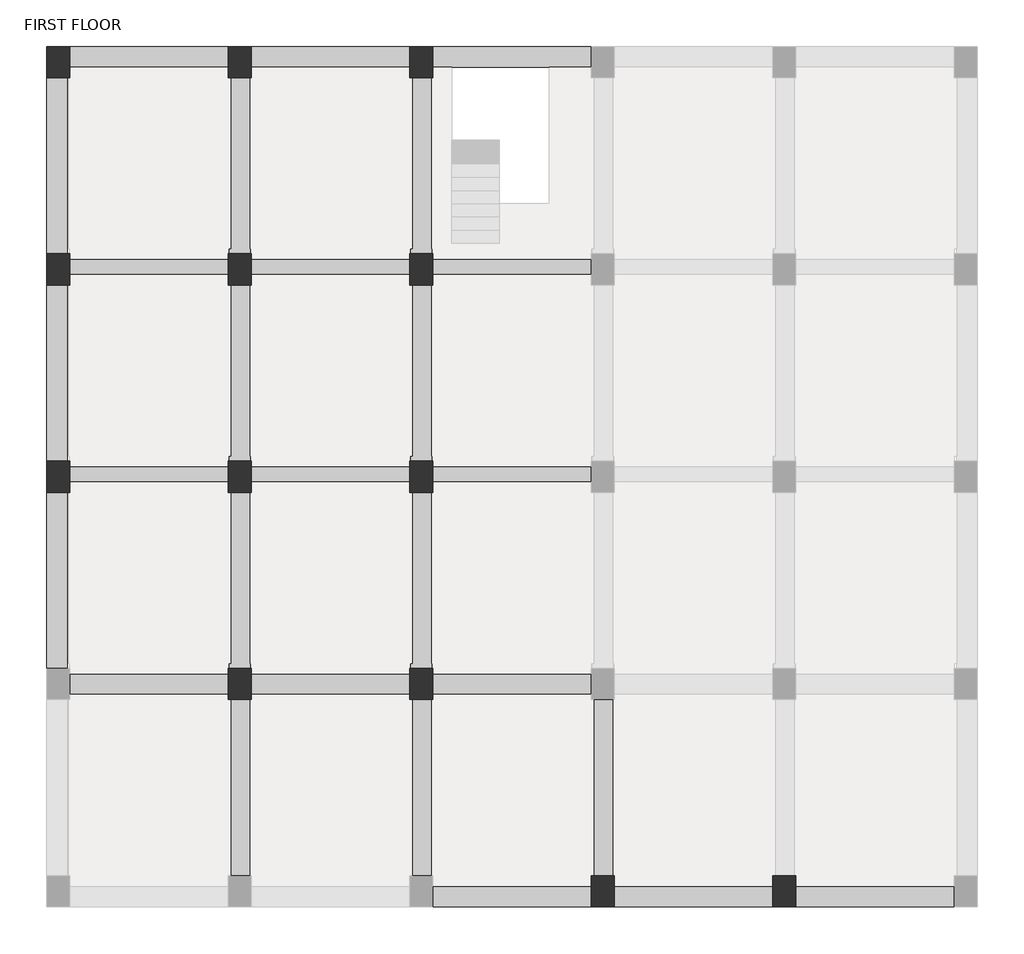
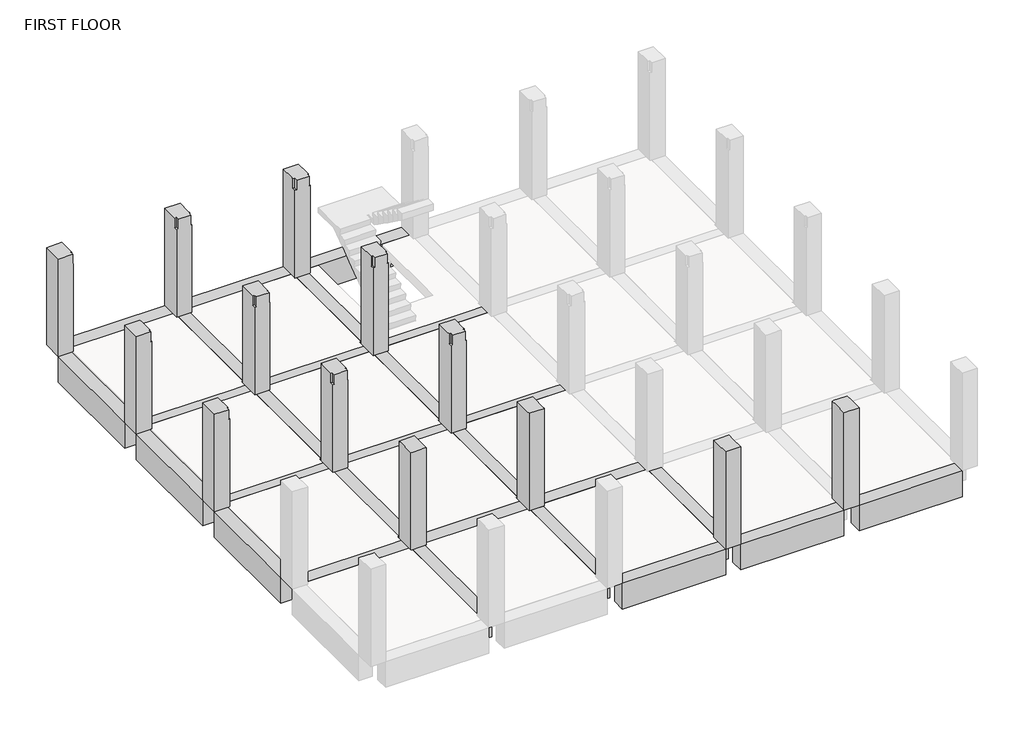
# One storey, part 3 of 4: 27 beams, 13 columns.
"""IFC4 building model written with IfcOpenShell, lengths in millimetres."""

from ifc_helpers import new_model, si_unit, frame, origin, place, context, project, spatial, polyline, outline, extrude, faceted_brep, element, save

model = new_model("IFC4")

# Units and contexts
model_context = context("Model", 3, world=origin())
ifc_project = project(units=[si_unit("LENGTHUNIT", "METRE", prefix="MILLI")], contexts=[model_context])

# Site, building, storey
site = spatial("IfcSite", under=ifc_project)
building = spatial("IfcBuilding", under=site)
storey = spatial("IfcBuildingStorey", under=building, Name="FIRST FLOOR", Elevation=3048.0)

# Beams
placement = place(None, origin())
element("IfcBeam", 1, ObjectType="M_Concrete-Rectangular Beam : 400 x 800mm", at=placement, inside=storey, context=model_context, shape_type="Brep", body=[
    faceted_brep([(4855.1115906, 3503.1212443, 3048.0), (4855.1115906, 3103.1212443, 3048.0), (7905.1115906, 3103.1212443, 3048.0), (7905.1115906, 3503.1212443, 3048.0), (4855.1115906, 3503.1212443, 2248.0), (4855.1115906, 3503.1212443, 2748.0), (7905.1115906, 3503.1212443, 2748.0), (7905.1115906, 3503.1212443, 2248.0), (4855.1115906, 3103.1212443, 2248.0), (7905.1115906, 3103.1212443, 2248.0)], [[[0, 1, 2, 3]], [[4, 5, 0, 3, 6, 7]], [[8, 4, 7, 9]], [[1, 8, 9, 2]], [[1, 0, 5, 4, 8]], [[3, 2, 9, 7, 6]]]),
])
element("IfcBeam", 2, ObjectType="M_Concrete-Rectangular Beam : 400 x 800mm", at=placement, inside=storey, context=model_context, shape_type="Brep", body=[
    faceted_brep([(1355.1115906, 3503.1212443, 3048.0), (1355.1115906, 3103.1212443, 3048.0), (4405.1115906, 3103.1212443, 3048.0), (4405.1115906, 3503.1212443, 3048.0), (1355.1115906, 3503.1212443, 2248.0), (1355.1115906, 3503.1212443, 2748.0), (4405.1115906, 3503.1212443, 2748.0), (4405.1115906, 3503.1212443, 2248.0), (1355.1115906, 3103.1212443, 2248.0), (4405.1115906, 3103.1212443, 2248.0)], [[[0, 1, 2, 3]], [[4, 5, 0, 3, 6, 7]], [[8, 4, 7, 9]], [[1, 8, 9, 2]], [[1, 0, 5, 4, 8]], [[3, 2, 9, 7, 6]]]),
])
element("IfcBeam", 3, ObjectType="M_Concrete-Rectangular Beam : 400 x 800mm", at=placement, inside=storey, context=model_context, shape_type="Brep", body=[
    faceted_brep([(-2144.8884094, 3503.1212443, 3048.0), (-2144.8884094, 3103.1212443, 3048.0), (905.1115906, 3103.1212443, 3048.0), (905.1115906, 3503.1212443, 3048.0), (-2144.8884094, 3503.1212443, 2248.0), (-2144.8884094, 3503.1212443, 2748.0), (905.1115906, 3503.1212443, 2748.0), (905.1115906, 3503.1212443, 2248.0), (-2144.8884094, 3103.1212443, 2248.0), (905.1115906, 3103.1212443, 2248.0)], [[[0, 1, 2, 3]], [[4, 5, 0, 3, 6, 7]], [[8, 4, 7, 9]], [[1, 8, 9, 2]], [[1, 0, 5, 4, 8]], [[3, 2, 9, 7, 6]]]),
])
element("IfcBeam", 4, ObjectType="M_Concrete-Rectangular Beam : 400 x 800mm", at=placement, inside=storey, context=model_context, shape_type="SweptSolid", body=[
    extrude(outline(polyline([(-9594.8884094, 11103.1212443), (-9194.8884094, 11103.1212443), (-9194.8884094, 7703.1212443), (-9594.8884094, 7703.1212443), (-9594.8884094, 11103.1212443)])), frame((0.0, 0.0, 2248.0), z_axis=(0.0, 0.0, 1.0), x_axis=(1.0, 0.0, 0.0)), (0.0, 0.0, 1.0), 800.0),
])
element("IfcBeam", 5, ObjectType="M_Concrete-Rectangular Beam : 400 x 800mm", at=placement, inside=storey, context=model_context, shape_type="SweptSolid", body=[
    extrude(outline(polyline([(-9594.8884094, 15103.1212443), (-9194.8884094, 15103.1212443), (-9194.8884094, 11703.1212443), (-9594.8884094, 11703.1212443), (-9594.8884094, 15103.1212443)])), frame((0.0, 0.0, 2248.0), z_axis=(0.0, 0.0, 1.0), x_axis=(1.0, 0.0, 0.0)), (0.0, 0.0, 1.0), 800.0),
])
element("IfcBeam", 6, ObjectType="M_Concrete-Rectangular Beam : 400 x 800mm", at=placement, inside=storey, context=model_context, shape_type="Brep", body=[
    faceted_brep([(-2594.8884094, 19303.1212443, 3048.0), (-2594.8884094, 19703.1212443, 3048.0), (-5644.8884094, 19703.1212443, 3048.0), (-5644.8884094, 19303.1212443, 3048.0), (-2594.8884094, 19303.1212443, 2248.0), (-2594.8884094, 19303.1212443, 2748.0), (-5644.8884094, 19303.1212443, 2748.0), (-5644.8884094, 19303.1212443, 2248.0), (-2594.8884094, 19703.1212443, 2248.0), (-5644.8884094, 19703.1212443, 2248.0)], [[[0, 1, 2, 3]], [[4, 5, 0, 3, 6, 7]], [[8, 4, 7, 9]], [[1, 8, 9, 2]], [[1, 0, 5, 4, 8]], [[3, 2, 9, 7, 6]]]),
])
element("IfcBeam", 7, ObjectType="M_Concrete-Rectangular Beam : 400 x 800mm", at=placement, inside=storey, context=model_context, shape_type="Brep", body=[
    faceted_brep([(-2144.8884094, 19703.1212443, 3048.0), (-2144.8884094, 19303.1212443, 3048.0), (-1784.8884094, 19303.1212443, 3048.0), (94.7115906, 19303.1212443, 3048.0), (905.1115906, 19303.1212443, 3048.0), (905.1115906, 19703.1212443, 3048.0), (-2144.8884094, 19303.1212443, 2748.0), (-2144.8884094, 19303.1212443, 2248.0), (905.1115906, 19303.1212443, 2248.0), (905.1115906, 19303.1212443, 2748.0), (-2144.8884094, 19703.1212443, 2248.0), (905.1115906, 19703.1212443, 2248.0)], [[[0, 1, 2, 3, 4, 5]], [[1, 6, 7, 8, 9, 4, 3, 2]], [[7, 10, 11, 8]], [[10, 0, 5, 11]], [[1, 0, 10, 7, 6]], [[5, 4, 9, 8, 11]]]),
])
element("IfcBeam", 8, ObjectType="M_Concrete-Rectangular Beam : 400 x 800mm", at=placement, inside=storey, context=model_context, shape_type="Brep", body=[
    faceted_brep([(-5669.8884094, 15703.1212443, 3048.0), (-5669.8884094, 15803.1212443, 3048.0), (-5669.8884094, 19103.1212443, 3048.0), (-6044.8884094, 19103.1212443, 3048.0), (-6044.8884094, 15803.1212443, 3048.0), (-6069.8884094, 15803.1212443, 3048.0), (-6069.8884094, 15703.1212443, 3048.0), (-6069.8884094, 19103.1212443, 2248.0), (-6069.8884094, 15703.1212443, 2248.0), (-6069.8884094, 15803.1212443, 2748.0), (-6069.8884094, 19103.1212443, 2748.0), (-5669.8884094, 19103.1212443, 2248.0), (-5669.8884094, 15703.1212443, 2248.0), (-6044.8884094, 19103.1212443, 2748.0), (-6044.8884094, 15803.1212443, 2748.0)], [[[0, 1, 2, 3, 4, 5, 6]], [[7, 8, 6, 5, 9, 10]], [[7, 11, 12, 8]], [[11, 2, 1, 0, 12]], [[11, 7, 10, 13, 3, 2]], [[0, 6, 8, 12]], [[9, 14, 13, 10]], [[14, 4, 3, 13]], [[4, 14, 9, 5]]]),
])
element("IfcBeam", 9, ObjectType="M_Concrete-Rectangular Beam : 400 x 800mm", at=placement, inside=storey, context=model_context, shape_type="Brep", body=[
    faceted_brep([(-5669.8884094, 11703.1212443, 3048.0), (-5669.8884094, 11803.1212443, 3048.0), (-5669.8884094, 15103.1212443, 3048.0), (-6044.8884094, 15103.1212443, 3048.0), (-6044.8884094, 11803.1212443, 3048.0), (-6069.8884094, 11803.1212443, 3048.0), (-6069.8884094, 11703.1212443, 3048.0), (-6069.8884094, 15103.1212443, 2248.0), (-6069.8884094, 11703.1212443, 2248.0), (-6069.8884094, 11803.1212443, 2748.0), (-6069.8884094, 15103.1212443, 2748.0), (-5669.8884094, 15103.1212443, 2248.0), (-5669.8884094, 11703.1212443, 2248.0), (-6044.8884094, 15103.1212443, 2748.0), (-6044.8884094, 11803.1212443, 2748.0)], [[[0, 1, 2, 3, 4, 5, 6]], [[7, 8, 6, 5, 9, 10]], [[7, 11, 12, 8]], [[11, 2, 1, 0, 12]], [[11, 7, 10, 13, 3, 2]], [[0, 6, 8, 12]], [[9, 14, 13, 10]], [[14, 4, 3, 13]], [[4, 14, 9, 5]]]),
])
element("IfcBeam", 10, ObjectType="M_Concrete-Rectangular Beam : 400 x 800mm", at=placement, inside=storey, context=model_context, shape_type="Brep", body=[
    faceted_brep([(-5669.8884094, 7703.1212443, 3048.0), (-5669.8884094, 7803.1212443, 3048.0), (-5669.8884094, 11103.1212443, 3048.0), (-6044.8884094, 11103.1212443, 3048.0), (-6044.8884094, 7803.1212443, 3048.0), (-6069.8884094, 7803.1212443, 3048.0), (-6069.8884094, 7703.1212443, 3048.0), (-6069.8884094, 11103.1212443, 2248.0), (-6069.8884094, 7703.1212443, 2248.0), (-6069.8884094, 7803.1212443, 2748.0), (-6069.8884094, 11103.1212443, 2748.0), (-5669.8884094, 11103.1212443, 2248.0), (-5669.8884094, 7703.1212443, 2248.0), (-6044.8884094, 11103.1212443, 2748.0), (-6044.8884094, 7803.1212443, 2748.0)], [[[0, 1, 2, 3, 4, 5, 6]], [[7, 8, 6, 5, 9, 10]], [[8, 7, 11, 12]], [[2, 1, 0, 12, 11]], [[2, 11, 7, 10, 13, 3]], [[0, 6, 8, 12]], [[9, 14, 13, 10]], [[14, 4, 3, 13]], [[4, 14, 9, 5]]]),
])
element("IfcBeam", 11, ObjectType="M_Concrete-Rectangular Beam : 400 x 800mm", at=placement, inside=storey, context=model_context, shape_type="Brep", body=[
    faceted_brep([(-5669.8884094, 3703.1212443, 3048.0), (-5669.8884094, 7103.1212443, 3048.0), (-6044.8884094, 7103.1212443, 3048.0), (-6044.8884094, 3703.1212443, 3048.0), (-6069.8884094, 7103.1212443, 2248.0), (-6069.8884094, 3703.1212443, 2248.0), (-6069.8884094, 3703.1212443, 2748.0), (-6069.8884094, 7103.1212443, 2748.0), (-5669.8884094, 7103.1212443, 2248.0), (-5669.8884094, 3703.1212443, 2248.0), (-5669.8884094, 7103.1212443, 2748.0), (-5669.8884094, 3703.1212443, 2748.0), (-6044.8884094, 7103.1212443, 2748.0), (-6044.8884094, 3703.1212443, 2748.0)], [[[0, 1, 2, 3]], [[4, 5, 6, 7]], [[4, 8, 9, 5]], [[8, 10, 1, 0, 11, 9]], [[8, 4, 7, 12, 2, 1, 10]], [[5, 9, 11, 0, 3, 13, 6]], [[13, 12, 7, 6]], [[12, 13, 3, 2]]]),
])
element("IfcBeam", 12, ObjectType="M_Concrete-Rectangular Beam : 400 x 800mm", at=placement, inside=storey, context=model_context, shape_type="Brep", body=[
    faceted_brep([(-2169.8884094, 15703.1212443, 3048.0), (-2169.8884094, 15803.1212443, 3048.0), (-2169.8884094, 19103.1212443, 3048.0), (-2544.8884094, 19103.1212443, 3048.0), (-2544.8884094, 15803.1212443, 3048.0), (-2569.8884094, 15803.1212443, 3048.0), (-2569.8884094, 15703.1212443, 3048.0), (-2569.8884094, 19103.1212443, 2248.0), (-2569.8884094, 15703.1212443, 2248.0), (-2569.8884094, 15803.1212443, 2748.0), (-2569.8884094, 19103.1212443, 2748.0), (-2169.8884094, 19103.1212443, 2248.0), (-2169.8884094, 15703.1212443, 2248.0), (-2544.8884094, 19103.1212443, 2748.0), (-2544.8884094, 15803.1212443, 2748.0)], [[[0, 1, 2, 3, 4, 5, 6]], [[7, 8, 6, 5, 9, 10]], [[7, 11, 12, 8]], [[11, 2, 1, 0, 12]], [[11, 7, 10, 13, 3, 2]], [[0, 6, 8, 12]], [[9, 14, 13, 10]], [[14, 4, 3, 13]], [[4, 14, 9, 5]]]),
])
element("IfcBeam", 13, ObjectType="M_Concrete-Rectangular Beam : 400 x 800mm", at=placement, inside=storey, context=model_context, shape_type="Brep", body=[
    faceted_brep([(-2169.8884094, 11703.1212443, 3048.0), (-2169.8884094, 11803.1212443, 3048.0), (-2169.8884094, 15103.1212443, 3048.0), (-2544.8884094, 15103.1212443, 3048.0), (-2544.8884094, 11803.1212443, 3048.0), (-2569.8884094, 11803.1212443, 3048.0), (-2569.8884094, 11703.1212443, 3048.0), (-2569.8884094, 15103.1212443, 2248.0), (-2569.8884094, 11703.1212443, 2248.0), (-2569.8884094, 11803.1212443, 2748.0), (-2569.8884094, 15103.1212443, 2748.0), (-2169.8884094, 15103.1212443, 2248.0), (-2169.8884094, 11703.1212443, 2248.0), (-2544.8884094, 15103.1212443, 2748.0), (-2544.8884094, 11803.1212443, 2748.0)], [[[0, 1, 2, 3, 4, 5, 6]], [[7, 8, 6, 5, 9, 10]], [[8, 7, 11, 12]], [[2, 1, 0, 12, 11]], [[2, 11, 7, 10, 13, 3]], [[0, 6, 8, 12]], [[9, 14, 13, 10]], [[14, 4, 3, 13]], [[4, 14, 9, 5]]]),
])
element("IfcBeam", 14, ObjectType="M_Concrete-Rectangular Beam : 400 x 800mm", at=placement, inside=storey, context=model_context, shape_type="Brep", body=[
    faceted_brep([(-2169.8884094, 7703.1212443, 3048.0), (-2169.8884094, 7803.1212443, 3048.0), (-2169.8884094, 11103.1212443, 3048.0), (-2544.8884094, 11103.1212443, 3048.0), (-2544.8884094, 7803.1212443, 3048.0), (-2569.8884094, 7803.1212443, 3048.0), (-2569.8884094, 7703.1212443, 3048.0), (-2569.8884094, 11103.1212443, 2248.0), (-2569.8884094, 7703.1212443, 2248.0), (-2569.8884094, 7803.1212443, 2748.0), (-2569.8884094, 11103.1212443, 2748.0), (-2169.8884094, 11103.1212443, 2248.0), (-2169.8884094, 7703.1212443, 2248.0), (-2544.8884094, 11103.1212443, 2748.0), (-2544.8884094, 7803.1212443, 2748.0)], [[[0, 1, 2, 3, 4, 5, 6]], [[7, 8, 6, 5, 9, 10]], [[7, 11, 12, 8]], [[11, 2, 1, 0, 12]], [[2, 11, 7, 10, 13, 3]], [[0, 6, 8, 12]], [[9, 14, 13, 10]], [[14, 4, 3, 13]], [[4, 14, 9, 5]]]),
])
element("IfcBeam", 15, ObjectType="M_Concrete-Rectangular Beam : 400 x 800mm", at=placement, inside=storey, context=model_context, shape_type="Brep", body=[
    faceted_brep([(-2169.8884094, 3703.1212443, 3048.0), (-2169.8884094, 7103.1212443, 3048.0), (-2544.8884094, 7103.1212443, 3048.0), (-2544.8884094, 3703.1212443, 3048.0), (-2569.8884094, 7103.1212443, 2248.0), (-2569.8884094, 3703.1212443, 2248.0), (-2569.8884094, 3703.1212443, 2748.0), (-2569.8884094, 7103.1212443, 2748.0), (-2169.8884094, 7103.1212443, 2248.0), (-2169.8884094, 3703.1212443, 2248.0), (-2169.8884094, 7103.1212443, 2748.0), (-2169.8884094, 3703.1212443, 2748.0), (-2544.8884094, 7103.1212443, 2748.0), (-2544.8884094, 3703.1212443, 2748.0)], [[[0, 1, 2, 3]], [[4, 5, 6, 7]], [[4, 8, 9, 5]], [[8, 10, 1, 0, 11, 9]], [[8, 4, 7, 12, 2, 1, 10]], [[5, 9, 11, 0, 3, 13, 6]], [[13, 12, 7, 6]], [[12, 13, 3, 2]]]),
])
element("IfcBeam", 16, ObjectType="M_Concrete-Rectangular Beam : 400 x 800mm", at=placement, inside=storey, context=model_context, shape_type="Brep", body=[
    faceted_brep([(1330.1115906, 3703.1212443, 3048.0), (1330.1115906, 7103.1212443, 3048.0), (955.1115906, 7103.1212443, 3048.0), (955.1115906, 3703.1212443, 3048.0), (930.1115906, 7103.1212443, 2248.0), (930.1115906, 3703.1212443, 2248.0), (930.1115906, 3703.1212443, 2748.0), (930.1115906, 7103.1212443, 2748.0), (1330.1115906, 7103.1212443, 2248.0), (1330.1115906, 3703.1212443, 2248.0), (1330.1115906, 7103.1212443, 2748.0), (1330.1115906, 3703.1212443, 2748.0), (955.1115906, 7103.1212443, 2748.0), (955.1115906, 3703.1212443, 2748.0)], [[[0, 1, 2, 3]], [[4, 5, 6, 7]], [[4, 8, 9, 5]], [[8, 10, 1, 0, 11, 9]], [[8, 4, 7, 12, 2, 1, 10]], [[5, 9, 11, 0, 3, 13, 6]], [[13, 12, 7, 6]], [[12, 13, 3, 2]]]),
])
element("IfcBeam", 17, ObjectType="M_Concrete-Rectangular Beam : 400 x 800mm", at=placement, inside=storey, context=model_context, shape_type="Brep", body=[
    faceted_brep([(-6094.8884094, 15603.1212443, 3048.0), (-9144.8884094, 15603.1212443, 3048.0), (-9144.8884094, 15303.1212443, 3048.0), (-6094.8884094, 15303.1212443, 3048.0), (-9144.8884094, 15203.1212443, 2248.0), (-6094.8884094, 15203.1212443, 2248.0), (-6094.8884094, 15203.1212443, 2748.0), (-9144.8884094, 15203.1212443, 2748.0), (-9144.8884094, 15603.1212443, 2248.0), (-6094.8884094, 15603.1212443, 2248.0), (-9144.8884094, 15603.1212443, 2748.0), (-6094.8884094, 15603.1212443, 2748.0), (-9144.8884094, 15303.1212443, 2748.0), (-6094.8884094, 15303.1212443, 2748.0)], [[[0, 1, 2, 3]], [[4, 5, 6, 7]], [[4, 8, 9, 5]], [[8, 10, 1, 0, 11, 9]], [[8, 4, 7, 12, 2, 1, 10]], [[5, 9, 11, 0, 3, 13, 6]], [[13, 12, 7, 6]], [[12, 13, 3, 2]]]),
])
element("IfcBeam", 18, ObjectType="M_Concrete-Rectangular Beam : 400 x 800mm", at=placement, inside=storey, context=model_context, shape_type="Brep", body=[
    faceted_brep([(-2594.8884094, 15603.1212443, 3048.0), (-5644.8884094, 15603.1212443, 3048.0), (-5644.8884094, 15303.1212443, 3048.0), (-2594.8884094, 15303.1212443, 3048.0), (-5644.8884094, 15203.1212443, 2248.0), (-2594.8884094, 15203.1212443, 2248.0), (-2594.8884094, 15203.1212443, 2748.0), (-5644.8884094, 15203.1212443, 2748.0), (-5644.8884094, 15603.1212443, 2248.0), (-2594.8884094, 15603.1212443, 2248.0), (-5644.8884094, 15603.1212443, 2748.0), (-2594.8884094, 15603.1212443, 2748.0), (-5644.8884094, 15303.1212443, 2748.0), (-2594.8884094, 15303.1212443, 2748.0)], [[[0, 1, 2, 3]], [[4, 5, 6, 7]], [[4, 8, 9, 5]], [[8, 10, 1, 0, 11, 9]], [[8, 4, 7, 12, 2, 1, 10]], [[5, 9, 11, 0, 3, 13, 6]], [[13, 12, 7, 6]], [[12, 13, 3, 2]]]),
])
element("IfcBeam", 19, ObjectType="M_Concrete-Rectangular Beam : 400 x 800mm", at=placement, inside=storey, context=model_context, shape_type="Brep", body=[
    faceted_brep([(905.1115906, 15603.1212443, 3048.0), (-2144.8884094, 15603.1212443, 3048.0), (-2144.8884094, 15303.1212443, 3048.0), (905.1115906, 15303.1212443, 3048.0), (-2144.8884094, 15603.1212443, 2248.0), (-2144.8884094, 15603.1212443, 2748.0), (905.1115906, 15603.1212443, 2748.0), (905.1115906, 15603.1212443, 2248.0), (-2144.8884094, 15203.1212443, 2248.0), (905.1115906, 15203.1212443, 2248.0), (905.1115906, 15203.1212443, 2748.0), (-2144.8884094, 15203.1212443, 2748.0), (-2144.8884094, 15303.1212443, 2748.0), (905.1115906, 15303.1212443, 2748.0)], [[[0, 1, 2, 3]], [[4, 5, 1, 0, 6, 7]], [[8, 4, 7, 9]], [[8, 9, 10, 11]], [[1, 5, 4, 8, 11, 12, 2]], [[7, 6, 0, 3, 13, 10, 9]], [[13, 12, 11, 10]], [[12, 13, 3, 2]]]),
])
element("IfcBeam", 20, ObjectType="M_Concrete-Rectangular Beam : 400 x 800mm", at=placement, inside=storey, context=model_context, shape_type="Brep", body=[
    faceted_brep([(905.1115906, 11603.1212443, 3048.0), (-2144.8884094, 11603.1212443, 3048.0), (-2144.8884094, 11303.1212443, 3048.0), (905.1115906, 11303.1212443, 3048.0), (-2144.8884094, 11603.1212443, 2248.0), (-2144.8884094, 11603.1212443, 2748.0), (905.1115906, 11603.1212443, 2748.0), (905.1115906, 11603.1212443, 2248.0), (-2144.8884094, 11203.1212443, 2248.0), (905.1115906, 11203.1212443, 2248.0), (905.1115906, 11203.1212443, 2748.0), (-2144.8884094, 11203.1212443, 2748.0), (-2144.8884094, 11303.1212443, 2748.0), (905.1115906, 11303.1212443, 2748.0)], [[[0, 1, 2, 3]], [[4, 5, 1, 0, 6, 7]], [[8, 4, 7, 9]], [[8, 9, 10, 11]], [[1, 5, 4, 8, 11, 12, 2]], [[7, 6, 0, 3, 13, 10, 9]], [[13, 12, 11, 10]], [[12, 13, 3, 2]]]),
])
element("IfcBeam", 21, ObjectType="M_Concrete-Rectangular Beam : 400 x 800mm", at=placement, inside=storey, context=model_context, shape_type="Brep", body=[
    faceted_brep([(-2594.8884094, 11603.1212443, 3048.0), (-5644.8884094, 11603.1212443, 3048.0), (-5644.8884094, 11303.1212443, 3048.0), (-2594.8884094, 11303.1212443, 3048.0), (-5644.8884094, 11603.1212443, 2248.0), (-5644.8884094, 11603.1212443, 2748.0), (-2594.8884094, 11603.1212443, 2748.0), (-2594.8884094, 11603.1212443, 2248.0), (-5644.8884094, 11203.1212443, 2248.0), (-2594.8884094, 11203.1212443, 2248.0), (-2594.8884094, 11203.1212443, 2748.0), (-5644.8884094, 11203.1212443, 2748.0), (-5644.8884094, 11303.1212443, 2748.0), (-2594.8884094, 11303.1212443, 2748.0)], [[[0, 1, 2, 3]], [[4, 5, 1, 0, 6, 7]], [[8, 4, 7, 9]], [[8, 9, 10, 11]], [[1, 5, 4, 8, 11, 12, 2]], [[7, 6, 0, 3, 13, 10, 9]], [[13, 12, 11, 10]], [[12, 13, 3, 2]]]),
])
element("IfcBeam", 22, ObjectType="M_Concrete-Rectangular Beam : 400 x 800mm", at=placement, inside=storey, context=model_context, shape_type="Brep", body=[
    faceted_brep([(-6094.8884094, 11603.1212443, 3048.0), (-9144.8884094, 11603.1212443, 3048.0), (-9144.8884094, 11303.1212443, 3048.0), (-6094.8884094, 11303.1212443, 3048.0), (-9144.8884094, 11603.1212443, 2248.0), (-9144.8884094, 11603.1212443, 2748.0), (-6094.8884094, 11603.1212443, 2748.0), (-6094.8884094, 11603.1212443, 2248.0), (-9144.8884094, 11203.1212443, 2248.0), (-6094.8884094, 11203.1212443, 2248.0), (-6094.8884094, 11203.1212443, 2748.0), (-9144.8884094, 11203.1212443, 2748.0), (-9144.8884094, 11303.1212443, 2748.0), (-6094.8884094, 11303.1212443, 2748.0)], [[[0, 1, 2, 3]], [[4, 5, 1, 0, 6, 7]], [[8, 4, 7, 9]], [[8, 9, 10, 11]], [[1, 5, 4, 8, 11, 12, 2]], [[7, 6, 0, 3, 13, 10, 9]], [[13, 12, 11, 10]], [[12, 13, 3, 2]]]),
])
element("IfcBeam", 23, ObjectType="M_Concrete-Rectangular Beam : 400 x 800mm", at=placement, inside=storey, context=model_context, shape_type="Brep", body=[
    faceted_brep([(-9144.8884094, 7603.1212443, 3048.0), (-9144.8884094, 7203.1212443, 3048.0), (-6094.8884094, 7203.1212443, 3048.0), (-6094.8884094, 7603.1212443, 3048.0), (-9144.8884094, 7203.1212443, 2748.0), (-9144.8884094, 7203.1212443, 2248.0), (-6094.8884094, 7203.1212443, 2248.0), (-6094.8884094, 7203.1212443, 2748.0), (-9144.8884094, 7603.1212443, 2248.0), (-6094.8884094, 7603.1212443, 2248.0), (-9144.8884094, 7603.1212443, 2748.0), (-6094.8884094, 7603.1212443, 2748.0)], [[[0, 1, 2, 3]], [[1, 4, 5, 6, 7, 2]], [[5, 8, 9, 6]], [[8, 10, 0, 3, 11, 9]], [[1, 0, 10, 8, 5, 4]], [[3, 2, 7, 6, 9, 11]]]),
])
element("IfcBeam", 24, ObjectType="M_Concrete-Rectangular Beam : 400 x 800mm", at=placement, inside=storey, context=model_context, shape_type="Brep", body=[
    faceted_brep([(-5644.8884094, 7603.1212443, 3048.0), (-5644.8884094, 7203.1212443, 3048.0), (-2594.8884094, 7203.1212443, 3048.0), (-2594.8884094, 7603.1212443, 3048.0), (-5644.8884094, 7203.1212443, 2748.0), (-5644.8884094, 7203.1212443, 2248.0), (-2594.8884094, 7203.1212443, 2248.0), (-2594.8884094, 7203.1212443, 2748.0), (-5644.8884094, 7603.1212443, 2248.0), (-2594.8884094, 7603.1212443, 2248.0), (-5644.8884094, 7603.1212443, 2748.0), (-2594.8884094, 7603.1212443, 2748.0)], [[[0, 1, 2, 3]], [[1, 4, 5, 6, 7, 2]], [[5, 8, 9, 6]], [[8, 10, 0, 3, 11, 9]], [[1, 0, 10, 8, 5, 4]], [[3, 2, 7, 6, 9, 11]]]),
])
element("IfcBeam", 25, ObjectType="M_Concrete-Rectangular Beam : 400 x 800mm", at=placement, inside=storey, context=model_context, shape_type="Brep", body=[
    faceted_brep([(-2144.8884094, 7603.1212443, 3048.0), (-2144.8884094, 7203.1212443, 3048.0), (905.1115906, 7203.1212443, 3048.0), (905.1115906, 7603.1212443, 3048.0), (-2144.8884094, 7203.1212443, 2748.0), (-2144.8884094, 7203.1212443, 2248.0), (905.1115906, 7203.1212443, 2248.0), (905.1115906, 7203.1212443, 2748.0), (-2144.8884094, 7603.1212443, 2248.0), (905.1115906, 7603.1212443, 2248.0), (-2144.8884094, 7603.1212443, 2748.0), (905.1115906, 7603.1212443, 2748.0)], [[[0, 1, 2, 3]], [[1, 4, 5, 6, 7, 2]], [[5, 8, 9, 6]], [[8, 10, 0, 3, 11, 9]], [[1, 0, 10, 8, 5, 4]], [[3, 2, 7, 6, 9, 11]]]),
])
element("IfcBeam", 26, ObjectType="M_Concrete-Rectangular Beam : 400 x 800mm", at=placement, inside=storey, context=model_context, shape_type="SweptSolid", body=[
    extrude(outline(polyline([(-9594.8884094, 19103.1212443), (-9194.8884094, 19103.1212443), (-9194.8884094, 15703.1212443), (-9594.8884094, 15703.1212443), (-9594.8884094, 19103.1212443)])), frame((0.0, 0.0, 2248.0), z_axis=(0.0, 0.0, 1.0), x_axis=(1.0, 0.0, 0.0)), (0.0, 0.0, 1.0), 800.0),
])
element("IfcBeam", 27, ObjectType="M_Concrete-Rectangular Beam : 400 x 800mm", at=placement, inside=storey, context=model_context, shape_type="Brep", body=[
    faceted_brep([(-6094.8884094, 19303.1212443, 3048.0), (-6094.8884094, 19703.1212443, 3048.0), (-9144.8884094, 19703.1212443, 3048.0), (-9144.8884094, 19303.1212443, 3048.0), (-6094.8884094, 19303.1212443, 2248.0), (-6094.8884094, 19303.1212443, 2748.0), (-9144.8884094, 19303.1212443, 2748.0), (-9144.8884094, 19303.1212443, 2248.0), (-6094.8884094, 19703.1212443, 2248.0), (-9144.8884094, 19703.1212443, 2248.0)], [[[0, 1, 2, 3]], [[4, 5, 0, 3, 6, 7]], [[8, 4, 7, 9]], [[1, 8, 9, 2]], [[2, 9, 7, 6, 3]], [[1, 0, 5, 4, 8]]]),
])

# Columns
element("IfcColumn", 28, ObjectType="M_Concrete-Rectangular-Column : 450 x 600mm", at=placement, inside=storey, context=model_context, shape_type="Brep", body=[
    faceted_brep([(-9144.8884094, 19703.1212443, 3048.0), (-9144.8884094, 19103.1212443, 3048.0), (-9594.8884094, 19103.1212443, 3048.0), (-9594.8884094, 19703.1212443, 3048.0), (-9144.8884094, 19703.1212443, 6096.0), (-9144.8884094, 19303.1212443, 6096.0), (-9144.8884094, 19203.1212443, 6096.0), (-9144.8884094, 19203.1212443, 5796.0), (-9144.8884094, 19103.1212443, 5796.0), (-9169.8884094, 19103.1212443, 5796.0), (-9169.8884094, 19103.1212443, 6096.0), (-9594.8884094, 19103.1212443, 6096.0), (-9594.8884094, 19703.1212443, 6096.0), (-9169.8884094, 19203.1212443, 6096.0), (-9169.8884094, 19203.1212443, 5796.0)], [[[0, 1, 2, 3]], [[1, 0, 4, 5, 6, 7, 8]], [[2, 1, 8, 9, 10, 11]], [[3, 2, 11, 12]], [[0, 3, 12, 4]], [[12, 11, 10, 13, 6, 5, 4]], [[7, 14, 9, 8]], [[14, 13, 10, 9]], [[14, 7, 6, 13]]]),
])
element("IfcColumn", 29, ObjectType="M_Concrete-Rectangular-Column : 450 x 600mm", at=placement, inside=storey, context=model_context, shape_type="Brep", body=[
    faceted_brep([(-5644.8884094, 19703.1212443, 3048.0), (-5644.8884094, 19103.1212443, 3048.0), (-6094.8884094, 19103.1212443, 3048.0), (-6094.8884094, 19703.1212443, 3048.0), (-5644.8884094, 19703.1212443, 6096.0), (-5644.8884094, 19303.1212443, 6096.0), (-5644.8884094, 19203.1212443, 6096.0), (-5644.8884094, 19203.1212443, 5796.0), (-5644.8884094, 19103.1212443, 5796.0), (-5669.8884094, 19103.1212443, 5796.0), (-5669.8884094, 19103.1212443, 6096.0), (-6044.8884094, 19103.1212443, 6096.0), (-6044.8884094, 19103.1212443, 5796.0), (-6094.8884094, 19103.1212443, 5796.0), (-6094.8884094, 19203.1212443, 5796.0), (-6094.8884094, 19203.1212443, 6096.0), (-6094.8884094, 19303.1212443, 6096.0), (-6094.8884094, 19703.1212443, 6096.0), (-6044.8884094, 19203.1212443, 6096.0), (-5669.8884094, 19203.1212443, 6096.0), (-5669.8884094, 19203.1212443, 5796.0), (-6044.8884094, 19203.1212443, 5796.0)], [[[0, 1, 2, 3]], [[1, 0, 4, 5, 6, 7, 8]], [[2, 1, 8, 9, 10, 11, 12, 13]], [[3, 2, 13, 14, 15, 16, 17]], [[0, 3, 17, 4]], [[4, 17, 16, 15, 18, 11, 10, 19, 6, 5]], [[7, 20, 9, 8]], [[20, 19, 10, 9]], [[20, 7, 6, 19]], [[21, 14, 13, 12]], [[18, 21, 12, 11]], [[14, 21, 18, 15]]]),
])
element("IfcColumn", 30, ObjectType="M_Concrete-Rectangular-Column : 450 x 600mm", at=placement, inside=storey, context=model_context, shape_type="Brep", body=[
    faceted_brep([(-2144.8884094, 19703.1212443, 3048.0), (-2144.8884094, 19103.1212443, 3048.0), (-2594.8884094, 19103.1212443, 3048.0), (-2594.8884094, 19703.1212443, 3048.0), (-2144.8884094, 19703.1212443, 6096.0), (-2144.8884094, 19303.1212443, 6096.0), (-2144.8884094, 19203.1212443, 6096.0), (-2144.8884094, 19203.1212443, 5796.0), (-2144.8884094, 19103.1212443, 5796.0), (-2169.8884094, 19103.1212443, 5796.0), (-2169.8884094, 19103.1212443, 6096.0), (-2544.8884094, 19103.1212443, 6096.0), (-2544.8884094, 19103.1212443, 5796.0), (-2594.8884094, 19103.1212443, 5796.0), (-2594.8884094, 19203.1212443, 5796.0), (-2594.8884094, 19203.1212443, 6096.0), (-2594.8884094, 19303.1212443, 6096.0), (-2594.8884094, 19703.1212443, 6096.0), (-2544.8884094, 19203.1212443, 6096.0), (-2169.8884094, 19203.1212443, 6096.0), (-2169.8884094, 19203.1212443, 5796.0), (-2544.8884094, 19203.1212443, 5796.0)], [[[0, 1, 2, 3]], [[1, 0, 4, 5, 6, 7, 8]], [[2, 1, 8, 9, 10, 11, 12, 13]], [[3, 2, 13, 14, 15, 16, 17]], [[0, 3, 17, 4]], [[4, 17, 16, 15, 18, 11, 10, 19, 6, 5]], [[7, 20, 9, 8]], [[20, 19, 10, 9]], [[20, 7, 6, 19]], [[21, 14, 13, 12]], [[18, 21, 12, 11]], [[14, 21, 18, 15]]]),
])
element("IfcColumn", 31, ObjectType="M_Concrete-Rectangular-Column : 450 x 600mm", at=placement, inside=storey, context=model_context, shape_type="Brep", body=[
    faceted_brep([(-9144.8884094, 15703.1212443, 3048.0), (-9144.8884094, 15103.1212443, 3048.0), (-9594.8884094, 15103.1212443, 3048.0), (-9594.8884094, 15703.1212443, 3048.0), (-9144.8884094, 15703.1212443, 5796.0), (-9144.8884094, 15703.1212443, 6096.0), (-9144.8884094, 15603.1212443, 6096.0), (-9144.8884094, 15303.1212443, 6096.0), (-9144.8884094, 15203.1212443, 6096.0), (-9144.8884094, 15203.1212443, 5796.0), (-9144.8884094, 15103.1212443, 5796.0), (-9169.8884094, 15103.1212443, 5796.0), (-9169.8884094, 15103.1212443, 6096.0), (-9594.8884094, 15103.1212443, 6096.0), (-9594.8884094, 15703.1212443, 6096.0), (-9169.8884094, 15203.1212443, 6096.0), (-9169.8884094, 15203.1212443, 5796.0)], [[[0, 1, 2, 3]], [[1, 0, 4, 5, 6, 7, 8, 9, 10]], [[2, 1, 10, 11, 12, 13]], [[3, 2, 13, 14]], [[0, 3, 14, 5, 4]], [[14, 13, 12, 15, 8, 7, 6, 5]], [[9, 16, 11, 10]], [[16, 15, 12, 11]], [[16, 9, 8, 15]]]),
])
element("IfcColumn", 32, ObjectType="M_Concrete-Rectangular-Column : 450 x 600mm", at=placement, inside=storey, context=model_context, shape_type="Brep", body=[
    faceted_brep([(-5644.8884094, 15703.1212443, 3048.0), (-5644.8884094, 15103.1212443, 3048.0), (-6094.8884094, 15103.1212443, 3048.0), (-6094.8884094, 15703.1212443, 3048.0), (-5644.8884094, 15703.1212443, 5796.0), (-5644.8884094, 15703.1212443, 6096.0), (-5644.8884094, 15603.1212443, 6096.0), (-5644.8884094, 15303.1212443, 6096.0), (-5644.8884094, 15203.1212443, 6096.0), (-5644.8884094, 15203.1212443, 5796.0), (-5644.8884094, 15103.1212443, 5796.0), (-5669.8884094, 15103.1212443, 5796.0), (-5669.8884094, 15103.1212443, 6096.0), (-6044.8884094, 15103.1212443, 6096.0), (-6044.8884094, 15103.1212443, 5796.0), (-6094.8884094, 15103.1212443, 5796.0), (-6094.8884094, 15203.1212443, 5796.0), (-6094.8884094, 15203.1212443, 6096.0), (-6094.8884094, 15303.1212443, 6096.0), (-6094.8884094, 15603.1212443, 6096.0), (-6094.8884094, 15703.1212443, 6096.0), (-6094.8884094, 15703.1212443, 5796.0), (-6044.8884094, 15203.1212443, 6096.0), (-5669.8884094, 15203.1212443, 6096.0), (-6044.8884094, 15203.1212443, 5796.0), (-5669.8884094, 15203.1212443, 5796.0)], [[[0, 1, 2, 3]], [[1, 0, 4, 5, 6, 7, 8, 9, 10]], [[2, 1, 10, 11, 12, 13, 14, 15]], [[3, 2, 15, 16, 17, 18, 19, 20, 21]], [[0, 3, 21, 20, 5, 4]], [[5, 20, 19, 18, 17, 22, 13, 12, 23, 8, 7, 6]], [[24, 16, 15, 14]], [[22, 24, 14, 13]], [[16, 24, 22, 17]], [[9, 25, 11, 10]], [[25, 23, 12, 11]], [[25, 9, 8, 23]]]),
])
element("IfcColumn", 33, ObjectType="M_Concrete-Rectangular-Column : 450 x 600mm", at=placement, inside=storey, context=model_context, shape_type="Brep", body=[
    faceted_brep([(-2144.8884094, 15703.1212443, 3048.0), (-2144.8884094, 15103.1212443, 3048.0), (-2594.8884094, 15103.1212443, 3048.0), (-2594.8884094, 15703.1212443, 3048.0), (-2144.8884094, 15703.1212443, 5796.0), (-2144.8884094, 15703.1212443, 6096.0), (-2144.8884094, 15603.1212443, 6096.0), (-2144.8884094, 15303.1212443, 6096.0), (-2144.8884094, 15203.1212443, 6096.0), (-2144.8884094, 15203.1212443, 5796.0), (-2144.8884094, 15103.1212443, 5796.0), (-2169.8884094, 15103.1212443, 5796.0), (-2169.8884094, 15103.1212443, 6096.0), (-2544.8884094, 15103.1212443, 6096.0), (-2544.8884094, 15103.1212443, 5796.0), (-2594.8884094, 15103.1212443, 5796.0), (-2594.8884094, 15203.1212443, 5796.0), (-2594.8884094, 15203.1212443, 6096.0), (-2594.8884094, 15303.1212443, 6096.0), (-2594.8884094, 15603.1212443, 6096.0), (-2594.8884094, 15703.1212443, 6096.0), (-2594.8884094, 15703.1212443, 5796.0), (-2544.8884094, 15203.1212443, 6096.0), (-2169.8884094, 15203.1212443, 6096.0), (-2169.8884094, 15203.1212443, 5796.0), (-2544.8884094, 15203.1212443, 5796.0)], [[[0, 1, 2, 3]], [[1, 0, 4, 5, 6, 7, 8, 9, 10]], [[2, 1, 10, 11, 12, 13, 14, 15]], [[3, 2, 15, 16, 17, 18, 19, 20, 21]], [[0, 3, 21, 20, 5, 4]], [[5, 20, 19, 18, 17, 22, 13, 12, 23, 8, 7, 6]], [[9, 24, 11, 10]], [[24, 23, 12, 11]], [[24, 9, 8, 23]], [[25, 16, 15, 14]], [[22, 25, 14, 13]], [[16, 25, 22, 17]]]),
])
element("IfcColumn", 34, ObjectType="M_Concrete-Rectangular-Column : 450 x 600mm", at=placement, inside=storey, context=model_context, shape_type="Brep", body=[
    faceted_brep([(-9144.8884094, 11703.1212443, 3048.0), (-9144.8884094, 11103.1212443, 3048.0), (-9594.8884094, 11103.1212443, 3048.0), (-9594.8884094, 11703.1212443, 3048.0), (-9144.8884094, 11703.1212443, 5796.0), (-9144.8884094, 11703.1212443, 6096.0), (-9144.8884094, 11603.1212443, 6096.0), (-9144.8884094, 11303.1212443, 6096.0), (-9144.8884094, 11203.1212443, 6096.0), (-9144.8884094, 11203.1212443, 5796.0), (-9144.8884094, 11103.1212443, 5796.0), (-9169.8884094, 11103.1212443, 5796.0), (-9169.8884094, 11103.1212443, 6096.0), (-9594.8884094, 11103.1212443, 6096.0), (-9594.8884094, 11703.1212443, 6096.0), (-9169.8884094, 11203.1212443, 6096.0), (-9169.8884094, 11203.1212443, 5796.0)], [[[0, 1, 2, 3]], [[1, 0, 4, 5, 6, 7, 8, 9, 10]], [[2, 1, 10, 11, 12, 13]], [[3, 2, 13, 14]], [[0, 3, 14, 5, 4]], [[14, 13, 12, 15, 8, 7, 6, 5]], [[9, 16, 11, 10]], [[16, 15, 12, 11]], [[16, 9, 8, 15]]]),
])
element("IfcColumn", 35, ObjectType="M_Concrete-Rectangular-Column : 450 x 600mm", at=placement, inside=storey, context=model_context, shape_type="Brep", body=[
    faceted_brep([(-5644.8884094, 11703.1212443, 3048.0), (-5644.8884094, 11103.1212443, 3048.0), (-6094.8884094, 11103.1212443, 3048.0), (-6094.8884094, 11703.1212443, 3048.0), (-5644.8884094, 11703.1212443, 5796.0), (-5644.8884094, 11703.1212443, 6096.0), (-5644.8884094, 11603.1212443, 6096.0), (-5644.8884094, 11303.1212443, 6096.0), (-5644.8884094, 11203.1212443, 6096.0), (-5644.8884094, 11203.1212443, 5796.0), (-5644.8884094, 11103.1212443, 5796.0), (-5669.8884094, 11103.1212443, 5796.0), (-5669.8884094, 11103.1212443, 6096.0), (-6044.8884094, 11103.1212443, 6096.0), (-6044.8884094, 11103.1212443, 5796.0), (-6094.8884094, 11103.1212443, 5796.0), (-6094.8884094, 11203.1212443, 5796.0), (-6094.8884094, 11203.1212443, 6096.0), (-6094.8884094, 11303.1212443, 6096.0), (-6094.8884094, 11603.1212443, 6096.0), (-6094.8884094, 11703.1212443, 6096.0), (-6094.8884094, 11703.1212443, 5796.0), (-6044.8884094, 11203.1212443, 6096.0), (-5669.8884094, 11203.1212443, 6096.0), (-5669.8884094, 11203.1212443, 5796.0), (-6044.8884094, 11203.1212443, 5796.0)], [[[0, 1, 2, 3]], [[1, 0, 4, 5, 6, 7, 8, 9, 10]], [[2, 1, 10, 11, 12, 13, 14, 15]], [[3, 2, 15, 16, 17, 18, 19, 20, 21]], [[0, 3, 21, 20, 5, 4]], [[5, 20, 19, 18, 17, 22, 13, 12, 23, 8, 7, 6]], [[9, 24, 11, 10]], [[24, 23, 12, 11]], [[24, 9, 8, 23]], [[25, 16, 15, 14]], [[22, 25, 14, 13]], [[16, 25, 22, 17]]]),
])
element("IfcColumn", 36, ObjectType="M_Concrete-Rectangular-Column : 450 x 600mm", at=placement, inside=storey, context=model_context, shape_type="Brep", body=[
    faceted_brep([(-2144.8884094, 11703.1212443, 3048.0), (-2144.8884094, 11103.1212443, 3048.0), (-2594.8884094, 11103.1212443, 3048.0), (-2594.8884094, 11703.1212443, 3048.0), (-2144.8884094, 11703.1212443, 5796.0), (-2144.8884094, 11703.1212443, 6096.0), (-2144.8884094, 11603.1212443, 6096.0), (-2144.8884094, 11303.1212443, 6096.0), (-2144.8884094, 11203.1212443, 6096.0), (-2144.8884094, 11203.1212443, 5796.0), (-2144.8884094, 11103.1212443, 5796.0), (-2169.8884094, 11103.1212443, 5796.0), (-2169.8884094, 11103.1212443, 6096.0), (-2544.8884094, 11103.1212443, 6096.0), (-2544.8884094, 11103.1212443, 5796.0), (-2594.8884094, 11103.1212443, 5796.0), (-2594.8884094, 11203.1212443, 5796.0), (-2594.8884094, 11203.1212443, 6096.0), (-2594.8884094, 11303.1212443, 6096.0), (-2594.8884094, 11603.1212443, 6096.0), (-2594.8884094, 11703.1212443, 6096.0), (-2594.8884094, 11703.1212443, 5796.0), (-2544.8884094, 11203.1212443, 6096.0), (-2169.8884094, 11203.1212443, 6096.0), (-2169.8884094, 11203.1212443, 5796.0), (-2544.8884094, 11203.1212443, 5796.0)], [[[0, 1, 2, 3]], [[1, 0, 4, 5, 6, 7, 8, 9, 10]], [[2, 1, 10, 11, 12, 13, 14, 15]], [[3, 2, 15, 16, 17, 18, 19, 20, 21]], [[0, 3, 21, 20, 5, 4]], [[5, 20, 19, 18, 17, 22, 13, 12, 23, 8, 7, 6]], [[9, 24, 11, 10]], [[24, 23, 12, 11]], [[24, 9, 8, 23]], [[25, 16, 15, 14]], [[22, 25, 14, 13]], [[16, 25, 22, 17]]]),
])
element("IfcColumn", 37, ObjectType="M_Concrete-Rectangular-Column : 450 x 600mm", at=placement, inside=storey, context=model_context, shape_type="Brep", body=[
    faceted_brep([(-5644.8884094, 7703.1212443, 3048.0), (-5644.8884094, 7103.1212443, 3048.0), (-6094.8884094, 7103.1212443, 3048.0), (-6094.8884094, 7703.1212443, 3048.0), (-5644.8884094, 7703.1212443, 5796.0), (-5644.8884094, 7703.1212443, 6096.0), (-5644.8884094, 7603.1212443, 6096.0), (-5644.8884094, 7203.1212443, 6096.0), (-5644.8884094, 7103.1212443, 6096.0), (-5644.8884094, 7103.1212443, 5796.0), (-5669.8884094, 7103.1212443, 6096.0), (-6044.8884094, 7103.1212443, 6096.0), (-6094.8884094, 7103.1212443, 6096.0), (-6094.8884094, 7103.1212443, 5796.0), (-6094.8884094, 7203.1212443, 6096.0), (-6094.8884094, 7603.1212443, 6096.0), (-6094.8884094, 7703.1212443, 6096.0), (-6094.8884094, 7703.1212443, 5796.0)], [[[0, 1, 2, 3]], [[1, 0, 4, 5, 6, 7, 8, 9]], [[2, 1, 9, 8, 10, 11, 12, 13]], [[3, 2, 13, 12, 14, 15, 16, 17]], [[0, 3, 17, 16, 5, 4]], [[5, 16, 15, 14, 12, 11, 10, 8, 7, 6]]]),
])
element("IfcColumn", 38, ObjectType="M_Concrete-Rectangular-Column : 450 x 600mm", at=placement, inside=storey, context=model_context, shape_type="Brep", body=[
    faceted_brep([(-2144.8884094, 7703.1212443, 3048.0), (-2144.8884094, 7103.1212443, 3048.0), (-2594.8884094, 7103.1212443, 3048.0), (-2594.8884094, 7703.1212443, 3048.0), (-2144.8884094, 7703.1212443, 5796.0), (-2144.8884094, 7703.1212443, 6096.0), (-2144.8884094, 7603.1212443, 6096.0), (-2144.8884094, 7203.1212443, 6096.0), (-2144.8884094, 7103.1212443, 6096.0), (-2144.8884094, 7103.1212443, 5796.0), (-2169.8884094, 7103.1212443, 6096.0), (-2544.8884094, 7103.1212443, 6096.0), (-2594.8884094, 7103.1212443, 6096.0), (-2594.8884094, 7103.1212443, 5796.0), (-2594.8884094, 7203.1212443, 6096.0), (-2594.8884094, 7603.1212443, 6096.0), (-2594.8884094, 7703.1212443, 6096.0), (-2594.8884094, 7703.1212443, 5796.0)], [[[0, 1, 2, 3]], [[1, 0, 4, 5, 6, 7, 8, 9]], [[2, 1, 9, 8, 10, 11, 12, 13]], [[3, 2, 13, 12, 14, 15, 16, 17]], [[0, 3, 17, 16, 5, 4]], [[5, 16, 15, 14, 12, 11, 10, 8, 7, 6]]]),
])
element("IfcColumn", 39, ObjectType="M_Concrete-Rectangular-Column : 450 x 600mm", at=placement, inside=storey, context=model_context, shape_type="Brep", body=[
    faceted_brep([(1355.1115906, 3703.1212443, 3048.0), (1355.1115906, 3103.1212443, 3048.0), (905.1115906, 3103.1212443, 3048.0), (905.1115906, 3703.1212443, 3048.0), (1355.1115906, 3703.1212443, 5796.0), (1355.1115906, 3703.1212443, 6096.0), (1355.1115906, 3503.1212443, 6096.0), (1355.1115906, 3103.1212443, 6096.0), (905.1115906, 3103.1212443, 6096.0), (905.1115906, 3503.1212443, 6096.0), (905.1115906, 3703.1212443, 6096.0), (905.1115906, 3703.1212443, 5796.0), (955.1115906, 3703.1212443, 6096.0), (1330.1115906, 3703.1212443, 6096.0)], [[[0, 1, 2, 3]], [[1, 0, 4, 5, 6, 7]], [[2, 1, 7, 8]], [[3, 2, 8, 9, 10, 11]], [[0, 3, 11, 10, 12, 13, 5, 4]], [[8, 7, 6, 5, 13, 12, 10, 9]]]),
])
element("IfcColumn", 40, ObjectType="M_Concrete-Rectangular-Column : 450 x 600mm", at=placement, inside=storey, context=model_context, shape_type="Brep", body=[
    faceted_brep([(4855.1115906, 3703.1212443, 3048.0), (4855.1115906, 3103.1212443, 3048.0), (4405.1115906, 3103.1212443, 3048.0), (4405.1115906, 3703.1212443, 3048.0), (4855.1115906, 3703.1212443, 5796.0), (4855.1115906, 3703.1212443, 6096.0), (4855.1115906, 3503.1212443, 6096.0), (4855.1115906, 3103.1212443, 6096.0), (4405.1115906, 3103.1212443, 6096.0), (4405.1115906, 3503.1212443, 6096.0), (4405.1115906, 3703.1212443, 6096.0), (4405.1115906, 3703.1212443, 5796.0), (4455.1115906, 3703.1212443, 6096.0), (4830.1115906, 3703.1212443, 6096.0)], [[[0, 1, 2, 3]], [[1, 0, 4, 5, 6, 7]], [[2, 1, 7, 8]], [[3, 2, 8, 9, 10, 11]], [[0, 3, 11, 10, 12, 13, 5, 4]], [[8, 7, 6, 5, 13, 12, 10, 9]]]),
])

save(model, "model.ifc")

# Revit data of these elements
# Type "M_Concrete-Rectangular Beam : 400 x 800mm"
#   Length [instance default] = 5' - 0"
#   b = 1' - 3.74803"
#   h = 2' - 7.49606"
#   Structural Material [instance default] = Concrete, Cast-in-Place gray
#   Assembly Code = ""
# Type "M_Concrete-Rectangular-Column : 450 x 600mm"
#   b = 1' - 5.71654"
#   h = 1' - 11.62205"
#   Structural Material [instance default] = Concrete, Cast-in-Place gray
# Elements 1, 2, 3, 4, 5, 6, 7, 8, 9, 10, 11, 12, 13, 14, 15, 16, 17, 18, 19, 20, 21, 22, 23, 24, 25, 26, 27 (IfcBeam, "M_Concrete-Rectangular Beam : 400 x 800mm")
#   Structural Material = Concrete, Cast-in-Place gray
#   Phase Created = New Construction
#   Materials on its faces: "Concrete, Cast-in-Place gray"
# Elements 28, 29, 30, 31, 32, 33, 34, 35, 36, 37, 38, 39, 40 (IfcColumn, "M_Concrete-Rectangular-Column : 450 x 600mm")
#   Structural Material = Concrete, Cast-in-Place gray
#   Phase Created = New Construction
#   Materials on its faces: "Concrete, Cast-in-Place gray"
# Materials
#   "Concrete, Cast-in-Place gray": class "Concrete", colour RGB 192 192 192, transparency 0, Description = "Cast-in-place concrete", Cost = 0
